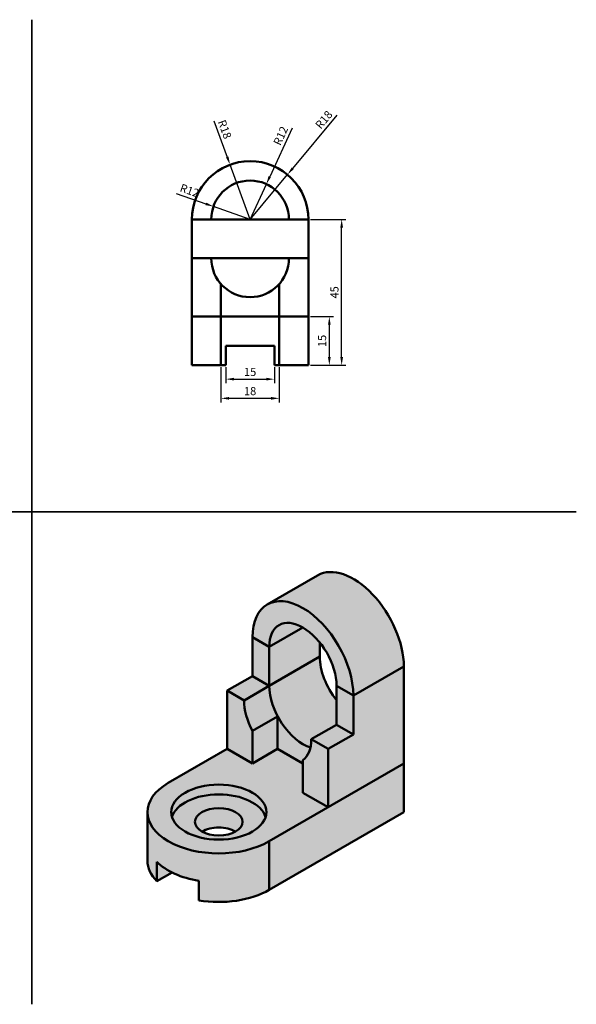
# Model space of a CAD drawing. Units: millimetres. Extents: x 2643 to 3341, y 1496 to 1804.
# Tile 1 of 2: x 2815 to 2987, y 1500 to 1804. Entities that reach past the tile are written whole.
import ezdxf

# ---------------------------------------------------------------- set-up
doc = ezdxf.new("R2010")
doc.units = ezdxf.units.MM
for name, color, linetype, lineweight in [('M-DIMS', 2, 'Continuous', 25), ('M-HATC', 252, 'Continuous', 18), ('M-OUTL', 7, 'Continuous', 50), ('M-TTLB', 8, 'Continuous', 35)]:
    doc.layers.add(name, color=color, linetype=linetype, lineweight=lineweight)
doc.styles.get("Standard").update_dxf_attribs({"font": 'arial.ttf'})
doc.dimstyles.new('ISO-25', dxfattribs={"dimtxt": 2.5, "dimasz": 2.5, "dimexe": 1.25, "dimexo": 0.625, "dimtad": 1, "dimtxsty": 'Standard', "dimcen": 2.5, "dimadec": 0, "dimazin": 0, "dimtfac": 1, "dimtmove": 0, "dimatfit": 3, "dimfxl": 1, "dimarcsym": 0})

# ---------------------------------------------------------------- blocks, each defined once
blk = doc.blocks.new('*D8')
at = {"layer": 'Defpoints', "color": 0, "transparency": 16777216}
for p in [(2878.539861946249, 1697.12622113536), (2893.539861946249, 1697.12622113536), (2893.539861946249, 1692.828022005697)]:
    blk.add_point(p, dxfattribs=at)
at = {"layer": 'M-DIMS', "color": 0, "lineweight": -2, "transparency": 16777216}
for p, q in [((2878.539861946249, 1696.50122113536), (2878.539861946249, 1691.578022005697)), ((2893.539861946249, 1696.50122113536), (2893.539861946249, 1691.578022005697)), ((2881.039861946249, 1692.828022005697), (2891.039861946249, 1692.828022005697))]:
    blk.add_line(p, q, dxfattribs=at)
at = {"layer": 'M-DIMS', "color": 0, "transparency": 16777216}
for points in [[(2881.039861946249, 1693.244688672364), (2881.039861946249, 1692.41135533903), (2878.539861946249, 1692.828022005697)], [(2891.039861946249, 1693.244688672364), (2891.039861946249, 1692.41135533903), (2893.539861946249, 1692.828022005697)]]:
    blk.add_solid(points, dxfattribs=at)
at = {"layer": 'M-DIMS', "color": 0, "transparency": 16777216, "insert": (2886.039861946249, 1694.729454475001), "char_height": 2.5, "attachment_point": 5}
blk.add_mtext('15', dxfattribs=at)
blk = doc.blocks.new('*D9')
at = {"layer": 'Defpoints', "color": 0, "transparency": 16777216}
for p in [(2877.039861946249, 1697.12622113536), (2895.039861946249, 1697.12622113536), (2895.039861946249, 1686.907164766469)]:
    blk.add_point(p, dxfattribs=at)
at = {"layer": 'M-DIMS', "color": 0, "lineweight": -2, "transparency": 16777216}
for p, q in [((2877.039861946249, 1696.50122113536), (2877.039861946249, 1685.657164766469)), ((2895.039861946249, 1696.50122113536), (2895.039861946249, 1685.657164766469)), ((2879.539861946249, 1686.907164766469), (2892.539861946249, 1686.907164766469))]:
    blk.add_line(p, q, dxfattribs=at)
at = {"layer": 'M-DIMS', "color": 0, "transparency": 16777216}
for points in [[(2879.539861946249, 1687.323831433136), (2879.539861946249, 1686.490498099803), (2877.039861946249, 1686.907164766469)], [(2892.539861946249, 1687.323831433136), (2892.539861946249, 1686.490498099803), (2895.039861946249, 1686.907164766469)]]:
    blk.add_solid(points, dxfattribs=at)
at = {"layer": 'M-DIMS', "color": 0, "transparency": 16777216, "insert": (2886.039861946249, 1688.808597235774), "char_height": 2.5, "attachment_point": 5}
blk.add_mtext('18', dxfattribs=at)
blk = doc.blocks.new('*D10')
at = {"layer": 'Defpoints', "color": 0, "transparency": 16777216}
for p in [(2904.03986194625, 1712.126221135361), (2910.511864211038, 1712.126221135361), (2904.03986194625, 1697.126221135361)]:
    blk.add_point(p, dxfattribs=at)
at = {"layer": 'M-DIMS', "color": 0, "lineweight": -2, "transparency": 16777216}
for p, q in [((2904.66486194625, 1712.126221135361), (2911.761864211038, 1712.126221135361)), ((2910.511864211038, 1699.626221135361), (2910.511864211038, 1709.626221135361)), ((2904.66486194625, 1697.126221135361), (2911.761864211038, 1697.126221135361))]:
    blk.add_line(p, q, dxfattribs=at)
at = {"layer": 'M-DIMS', "color": 0, "transparency": 16777216}
for points in [[(2910.095197544371, 1709.626221135361), (2910.928530877704, 1709.626221135361), (2910.511864211038, 1712.126221135361)], [(2910.095197544371, 1699.626221135361), (2910.928530877704, 1699.626221135361), (2910.511864211038, 1697.126221135361)]]:
    blk.add_solid(points, dxfattribs=at)
at = {"layer": 'M-DIMS', "color": 0, "transparency": 16777216, "insert": (2908.610431741733, 1704.626221135359), "char_height": 2.5, "attachment_point": 5, "rotation": 90}
blk.add_mtext('15', dxfattribs=at)
blk = doc.blocks.new('*D11')
at = {"layer": 'Defpoints', "color": 0, "transparency": 16777216}
for p in [(2904.03986194625, 1742.126221135361), (2914.32004968833, 1742.126221135361), (2904.03986194625, 1697.126221135361)]:
    blk.add_point(p, dxfattribs=at)
at = {"layer": 'M-DIMS', "color": 0, "lineweight": -2, "transparency": 16777216}
for p, q in [((2904.66486194625, 1742.126221135361), (2915.57004968833, 1742.126221135361)), ((2914.32004968833, 1699.626221135361), (2914.32004968833, 1739.626221135361)), ((2904.66486194625, 1697.126221135361), (2915.57004968833, 1697.126221135361))]:
    blk.add_line(p, q, dxfattribs=at)
at = {"layer": 'M-DIMS', "color": 0, "transparency": 16777216}
for points in [[(2913.903383021663, 1739.626221135361), (2914.736716354996, 1739.626221135361), (2914.32004968833, 1742.126221135361)], [(2913.903383021663, 1699.626221135361), (2914.736716354996, 1699.626221135361), (2914.32004968833, 1697.126221135361)]]:
    blk.add_solid(points, dxfattribs=at)
at = {"layer": 'M-DIMS', "color": 0, "transparency": 16777216, "insert": (2912.423733180827, 1719.626221135359), "char_height": 2.5, "attachment_point": 5, "rotation": 90}
blk.add_mtext('45', dxfattribs=at)
blk = doc.blocks.new('*D12')
at = {"layer": 'Defpoints', "color": 0, "transparency": 16777216}
for p in [(2897.568460366327, 1755.9498031049), (2886.039861946246, 1742.126221135359)]:
    blk.add_point(p, dxfattribs=at)
at = {"layer": 'M-DIMS', "color": 0, "lineweight": -2, "transparency": 16777216}
for p, q in [((2912.838621649522, 1774.259776138453), (2899.169654591339, 1757.869745045113)), ((2886.039861946246, 1742.126221135359), (2897.568460366327, 1755.9498031049))]:
    blk.add_line(p, q, dxfattribs=at)
at = {"layer": 'M-DIMS', "color": 0, "transparency": 16777216}
blk.add_solid([(2898.849664267969, 1758.136610749282), (2899.489644914707, 1757.602879340945), (2897.568460366327, 1755.9498031049)], dxfattribs=at)
at = {"layer": 'M-DIMS', "color": 0, "transparency": 16777216, "insert": (2909.063405808288, 1772.701805209806), "char_height": 2.5, "attachment_point": 5, "rotation": 50.172551131776245}
blk.add_mtext('R18', dxfattribs=at)
blk = doc.blocks.new('*D13')
at = {"layer": 'Defpoints', "color": 0, "transparency": 16777216}
for p in [(2891.051977523317, 1753.029371938779), (2886.039861946248, 1742.126221135359)]:
    blk.add_point(p, dxfattribs=at)
at = {"layer": 'M-DIMS', "color": 0, "lineweight": -2, "transparency": 16777216}
for p, q in [((2898.991408479002, 1770.300484640011), (2892.09616826854, 1755.300861689492)), ((2886.039861946248, 1742.126221135359), (2891.051977523317, 1753.029371938779))]:
    blk.add_line(p, q, dxfattribs=at)
at = {"layer": 'M-DIMS', "color": 0, "transparency": 16777216}
blk.add_solid([(2891.717586643421, 1755.474893480363), (2892.474749893659, 1755.126829898622), (2891.051977523317, 1753.029371938779)], dxfattribs=at)
at = {"layer": 'M-DIMS', "color": 0, "transparency": 16777216, "insert": (2895.779892777806, 1767.815655975434), "char_height": 2.5, "attachment_point": 5, "rotation": 65.31203083876427}
blk.add_mtext('R12', dxfattribs=at)
blk = doc.blocks.new('*D35')
at = {"layer": 'Defpoints', "color": 0, "transparency": 16777216}
for p in [(2879.838123, 1759.024104), (2886.039862, 1742.126221)]:
    blk.add_point(p, dxfattribs=at)
at = {"layer": 'M-DIMS', "color": 0, "lineweight": -2, "transparency": 16777216}
for p, q in [((2874.871761228464, 1772.555953720068), (2878.976770383051, 1761.371032134664)), ((2886.039862, 1742.126221), (2879.838123, 1759.024104))]:
    blk.add_line(p, q, dxfattribs=at)
at = {"layer": 'M-DIMS', "color": 0, "transparency": 16777216}
blk.add_solid([(2879.367925072162, 1761.514590904155), (2878.585615693941, 1761.227473365172), (2879.838123, 1759.024104)], dxfattribs=at)
at = {"layer": 'M-DIMS', "color": 0, "transparency": 16777216, "insert": (2877.902089838132, 1769.817955075101), "char_height": 2.5, "attachment_point": 5, "rotation": 290.1537820808809}
blk.add_mtext('R18', dxfattribs=at)
blk = doc.blocks.new('*D36')
at = {"layer": 'Defpoints', "color": 0, "transparency": 16777216}
for p in [(2874.721666, 1746.113505), (2886.039862000001, 1742.126221)]:
    blk.add_point(p, dxfattribs=at)
at = {"layer": 'M-DIMS', "color": 0, "lineweight": -2, "transparency": 16777216}
for p, q in [((2863.216570279684, 1750.16663184849), (2872.363708454077, 1746.944189182844)), ((2886.039862000001, 1742.126221), (2874.721666, 1746.113505))]:
    blk.add_line(p, q, dxfattribs=at)
at = {"layer": 'M-DIMS', "color": 0, "transparency": 16777216}
blk.add_solid([(2872.502155817885, 1747.337182107165), (2872.22526109027, 1746.551196258524), (2874.721666, 1746.113505)], dxfattribs=at)
at = {"layer": 'M-DIMS', "color": 0, "transparency": 16777216, "insert": (2867.235873630472, 1750.744046054824), "char_height": 2.5, "attachment_point": 5, "rotation": 340.59316357138516}
blk.add_mtext('R12', dxfattribs=at)

msp = doc.modelspace()

# ---------------------------------------------------------------- hatches: boundary and pattern name
at = {"layer": 'M-HATC'}
h = msp.add_hatch(color=256, dxfattribs=at)
h.dxf.hatch_style = 1
h.paths.add_polyline_path([(2933.516942481301, 1604.176370603883), (2917.92848521322, 1595.176370603883), (2917.92848521322, 1583.176370603883), (2910.134256579122, 1578.676370603883), (2910.134256579238, 1560.676370603955), (2933.516942481301, 1574.176370603883)])
h.paths.add_polyline_path([(2933.516942481301, 1574.176370603883), (2910.134256579238, 1560.676370603955), (2891.947723099637, 1550.176370603883), (2891.947723099637, 1535.176370603883), (2933.516942481301, 1559.176370603883)])
edge = h.paths.add_edge_path()
edge.add_line((2910.134256579169, 1560.676370603914), (2902.340027945024, 1565.176370603942))
edge.add_line((2902.340027945024, 1565.176370603942), (2902.340027945024, 1574.176370604203))
edge.add_line((2902.340027945024, 1574.176370604203), (2894.545799311216, 1578.676370604033))
edge.add_line((2894.545799311216, 1578.676370604033), (2886.75157067706, 1574.176370603912))
edge.add_line((2886.75157067706, 1574.176370603912), (2878.957342042936, 1578.676370603927))
edge.add_line((2878.957342042936, 1578.676370603927), (2860.770808564148, 1568.176370604339))
edge.add_ellipse((2876.359265831439, 1559.176370603883), major_axis=(-22.04540768513047, 0), ratio=0.5773502691893942, start_angle=150.0000000000131, end_angle=329.99999999998147, ccw=False)
edge.add_line((2891.947723099778, 1550.176370603965), (2910.134256579169, 1560.676370603914))
edge = h.paths.add_edge_path()
edge.add_ellipse((2876.359265831439, 1559.176370603883), major_axis=(-22.04540768513047, 0), ratio=0.5773502691893942, start_angle=0, end_angle=150.0000000000124, ccw=False)
edge.add_line((2854.313858146337, 1559.176370603687), (2854.313858146337, 1544.176370603629))
edge.add_ellipse((2876.359265831439, 1544.176370603883), major_axis=(-22.04540768513047, 0), ratio=0.5773502691893942, start_angle=360, end_angle=378.3086229740257)
edge.add_line((2857.232362851408, 1537.847558645967), (2857.232362851408, 1543.847558645968))
edge.add_ellipse((2876.359265831439, 1550.176370603883), major_axis=(-22.04540768513047, 0), ratio=0.5773502691893942, start_angle=378.3086229740257, end_angle=393.6807393147395)
edge.add_ellipse((2876.359265831439, 1550.176370603883), major_axis=(-22.04540768513047, 0), ratio=0.5773502691893942, start_angle=393.6807393147395, end_angle=423.3447265862672)
edge.add_line((2870.222743908083, 1537.951490254265), (2870.222743908083, 1531.951490254265))
edge.add_ellipse((2876.359265831439, 1544.176370603883), major_axis=(-22.04540768513047, 0), ratio=0.5773502691893942, start_angle=423.3447265862672, end_angle=510.0000000000425)
edge.add_line((2891.947723099637, 1535.176370603864), (2891.947723099637, 1550.176370603863))
edge = h.paths.add_edge_path()
edge.add_ellipse((2876.359265831439, 1559.176370603883), major_axis=(-22.04540768513047, 0), ratio=0.5773502691893942, start_angle=0, end_angle=150.0000000000123)
edge.add_ellipse((2876.359265831439, 1559.176370603883), major_axis=(-22.04540768513047, 0), ratio=0.5773502691893942, start_angle=150.0000000000123, end_angle=329.9999999999814)
edge.add_ellipse((2876.359265831439, 1559.176370603883), major_axis=(-22.04540768513047, 0), ratio=0.5773502691893942, start_angle=329.9999999999814, end_angle=360)
edge = h.paths.add_edge_path(flags=16)
edge.add_ellipse((2876.359265831439, 1559.176370603883), major_axis=(-14.69693845669906, 0), ratio=0.5773502691902185, start_angle=5.920136941275302, end_angle=174.0798630587249, ccw=False)
edge.add_ellipse((2876.359265831439, 1559.176370603883), major_axis=(-14.69693845669906, 0), ratio=0.5773502691902185, start_angle=174.0798630587249, end_angle=365.92013694127525, ccw=False)
edge = h.paths.add_edge_path(flags=0)
edge.add_ellipse((2876.359265831439, 1556.176370603883), major_axis=(-7.348469228349532, 0), ratio=0.5773502691902185, start_angle=0, end_angle=360)
h.paths.add_polyline_path([(2894.545799311274, 1588.73911667028), (2886.75157067706, 1584.239116670192), (2886.75157067706, 1574.176370603912), (2894.545799311274, 1578.676370604067)])
edge = h.paths.add_edge_path()
edge.add_ellipse((2894.545799310925, 1587.676370603796), major_axis=(7.348469228327981, -12.72792206133827), ratio=0.5773502691919116, start_angle=210.0000000002129, end_angle=263.79747378773834, ccw=False)
edge.add_line((2884.153494465513, 1593.676370603782), (2878.957342042961, 1596.676370603883))
edge.add_line((2878.957342042961, 1596.676370603883), (2878.957342042961, 1578.676370603913))
edge.add_line((2878.957342042961, 1578.676370603913), (2886.75157067706, 1574.176370603912))
edge.add_line((2886.75157067706, 1574.176370603912), (2886.75157067706, 1584.2391166702))
edge = h.paths.add_edge_path()
edge.add_line((2910.134256579122, 1578.676370603883), (2904.938104156335, 1581.676370603783))
edge.add_ellipse((2894.545799310925, 1587.676370603796), major_axis=(7.348469228327981, -12.72792206133827), ratio=0.5773502691919116, start_angle=379.85756861646945, end_angle=389.9999999999722, ccw=False)
edge.add_ellipse((2894.545799310925, 1587.676370603796), major_axis=(7.348469228327981, -12.72792206133827), ratio=0.5773502691919116, start_angle=362.0747159111078, end_angle=379.85756861646945, ccw=False)
edge.add_line((2902.340027945024, 1575.239116670666), (2902.340027945024, 1565.176370603942))
edge.add_line((2902.340027945024, 1565.176370603942), (2910.134256579238, 1560.676370603874))
edge.add_line((2910.134256579238, 1560.676370603874), (2910.134256579122, 1578.676370603883))
h.paths.add_polyline_path([(2917.92848521322, 1583.176370603883), (2912.732332790527, 1586.176370603883), (2904.938104156304, 1581.676370603801), (2910.134256579122, 1578.676370603883)])
h.paths.add_polyline_path([(2891.947723099804, 1598.176370603854), (2886.75157067706, 1601.176370603883), (2878.957342042961, 1596.676370603883), (2884.153494465538, 1593.676370603767)])
h.paths.add_polyline_path([(2891.947723099753, 1610.176370603883), (2886.75157067706, 1613.176370603883), (2886.75157067706, 1601.176370603883), (2891.947723099753, 1598.176370603883)], flags=17)
edge = h.paths.add_edge_path()
edge.add_ellipse((2902.34002794514, 1604.176370603883), major_axis=(7.348469228327981, -12.72792206133827), ratio=0.5773502691919116, start_angle=510.0000000000128, end_angle=569.999999999972, ccw=False)
edge.add_ellipse((2902.34002794514, 1604.176370603883), major_axis=(7.348469228327981, -12.72792206133827), ratio=0.5773502691919116, start_angle=474.8960906392445, end_angle=510.0000000000128, ccw=False)
edge.add_ellipse((2902.34002794514, 1604.176370603883), major_axis=(7.348469228327981, -12.72792206133827), ratio=0.5773502691919116, start_angle=389.9999999999722, end_angle=474.8960906392445, ccw=False)
edge.add_line((2912.73233279055, 1598.17637060387), (2917.928485213233, 1595.176370603877))
edge.add_ellipse((2902.34002794514, 1604.176370603883), major_axis=(11.02270384251673, -19.09188309199311), ratio=0.5773502691892949, start_angle=29.99999999989788, end_angle=180.0000000000081)
edge.add_ellipse((2902.34002794514, 1604.176370603883), major_axis=(11.02270384251673, -19.09188309199311), ratio=0.5773502691892949, start_angle=180.0000000000081, end_angle=209.9999999998979)
edge.add_line((2886.751570677047, 1613.17637060389), (2891.947723099729, 1610.176370603897))
h.paths.add_polyline_path([(2917.92848521322, 1595.176370603883), (2912.732332790527, 1598.176370603883), (2912.732332790527, 1586.176370603883), (2917.92848521322, 1583.176370603883)], flags=17)
edge = h.paths.add_edge_path()
edge.add_ellipse((2917.92848521322, 1613.176370603883), major_axis=(11.02270384251673, -19.09188309199311), ratio=0.5773502691892949, start_angle=29.99999999989788, end_angle=180)
edge.add_line((2906.905781370834, 1632.268253695929), (2891.317324102751, 1623.268253695927))
edge.add_ellipse((2902.34002794514, 1604.176370603883), major_axis=(11.02270384251673, -19.09188309199311), ratio=0.5773502691892949, start_angle=29.99999999989791, end_angle=180.0000000000082, ccw=False)
edge.add_line((2917.928485213232, 1595.17637060389), (2933.516942481312, 1604.17637060389))
edge = h.paths.add_edge_path(flags=17)
edge.add_ellipse((2876.359265831439, 1550.176370603883), major_axis=(-22.04540768513047, 0), ratio=0.5773502691893942, start_angle=378.3086229740258, end_angle=393.6807393147396, ccw=False)
edge.add_line((2857.232362851408, 1543.847558645968), (2857.232362851408, 1537.847558645975))
edge.add_line((2857.232362851408, 1537.847558645975), (2861.92424961148, 1540.556420729916))
edge = h.paths.add_edge_path()
edge.add_ellipse((2894.545799310925, 1587.676370603796), major_axis=(7.348469228327981, -12.72792206133827), ratio=0.5773502691919116, start_angle=362.0747159111078, end_angle=379.8575686164694)
edge.add_ellipse((2902.34002794514, 1592.176370603883), major_axis=(7.348469228327981, -12.72792206133827), ratio=0.5773502691919116, start_angle=263.79747378769656, end_angle=340.14243138353595, ccw=False)
edge.add_line((2894.545799311274, 1588.739116670287), (2894.545799311274, 1578.676370604))
edge.add_line((2894.545799311274, 1578.676370604), (2902.340027945024, 1574.176370604203))
edge.add_line((2902.340027945024, 1574.176370604203), (2902.340027945024, 1575.239116670666))
h = msp.add_hatch(color=256, dxfattribs=at)
h.dxf.hatch_style = 1
edge = h.paths.add_edge_path()
edge.add_ellipse((2902.34002794514, 1592.176370603883), major_axis=(7.348469228327981, -12.72792206133827), ratio=0.5773502691919116, start_angle=210.0000000002129, end_angle=263.79747378769656, ccw=False)
edge.add_line((2891.947723099731, 1598.176370603812), (2884.153494465514, 1593.676370603753))
edge.add_ellipse((2894.545799310925, 1587.676370603796), major_axis=(7.348469228327981, -12.72792206133827), ratio=0.5773502691919116, start_angle=210.0000000002128, end_angle=263.7974737877383)
edge.add_line((2886.751570677063, 1584.239116670194), (2894.545799311277, 1588.739116670281))
edge = h.paths.add_edge_path()
edge.add_ellipse((2917.92848521322, 1601.176370603883), major_axis=(7.348469228327981, -12.72792206133827), ratio=0.5773502691919116, start_angle=210.0000000002129, end_angle=294.89609063918937, ccw=False)
edge.add_line((2907.53618036781, 1607.176370603841), (2891.947723099728, 1598.176370603869))
edge.add_ellipse((2902.34002794514, 1592.176370603883), major_axis=(7.348469228327981, -12.72792206133827), ratio=0.5773502691919116, start_angle=210.0000000002128, end_angle=263.7974737876965)
edge.add_ellipse((2902.34002794514, 1592.176370603883), major_axis=(7.348469228327981, -12.72792206133827), ratio=0.5773502691919116, start_angle=263.7974737876965, end_angle=340.142431383536)
edge.add_ellipse((2894.545799310925, 1587.676370603796), major_axis=(7.348469228327981, -12.72792206133827), ratio=0.5773502691919116, start_angle=379.8575686164694, end_angle=389.9999999999722)
edge.add_line((2904.938104156336, 1581.676370603819), (2912.732332790527, 1586.176370603883))
edge.add_line((2912.732332790527, 1586.176370603883), (2912.732332790527, 1593.784065758426))
edge = h.paths.add_edge_path()
edge.add_line((2907.536180367833, 1607.176370603854), (2907.536180367833, 1611.568675449341))
edge.add_ellipse((2902.34002794514, 1604.176370603883), major_axis=(7.348469228327981, -12.72792206133827), ratio=0.5773502691919116, start_angle=474.8960906392444, end_angle=510.0000000000128)
edge.add_line((2902.340027945145, 1616.176370603886), (2891.947723099753, 1610.176370603883))
edge.add_line((2891.947723099753, 1610.176370603883), (2891.947723099753, 1598.176370603883))
edge.add_line((2891.947723099753, 1598.176370603883), (2907.536180367833, 1607.176370603854))
edge = h.paths.add_edge_path()
edge.add_ellipse((2902.34002794514, 1604.176370603883), major_axis=(7.348469228327981, -12.72792206133827), ratio=0.5773502691919116, start_angle=510.0000000000128, end_angle=209.9999999999721)
edge.add_line((2891.947723099728, 1610.176370603869), (2902.340027945145, 1616.176370603886))
edge = h.paths.add_edge_path()
edge.add_ellipse((2876.359265831439, 1559.176370603883), major_axis=(-14.69693845669906, 0), ratio=0.5773502691902185, start_angle=174.0798630587248, end_angle=365.9201369412752)
edge.add_ellipse((2876.359265831439, 1556.176370603883), major_axis=(-14.69693845669906, 0), ratio=0.5773502691902185, start_angle=185.9201369408757, end_angle=354.0798630591243, ccw=False)
edge = h.paths.add_edge_path()
edge.add_ellipse((2876.359265831439, 1556.176370603883), major_axis=(-14.69693845669906, 0), ratio=0.5773502691902185, start_angle=185.9201369408757, end_angle=354.0798630591242)
edge.add_ellipse((2876.359265831439, 1559.176370603883), major_axis=(-14.69693845669906, 0), ratio=0.5773502691902185, start_angle=5.920136941275217, end_angle=174.0798630587248)
edge = h.paths.add_edge_path(flags=16)
edge.add_ellipse((2876.359265831439, 1556.176370603883), major_axis=(-7.348469228349532, 0), ratio=0.5773502691902185, start_angle=0, end_angle=360)
h = msp.add_hatch(color=256, dxfattribs=at)
h.dxf.hatch_style = 1
edge = h.paths.add_edge_path()
edge.add_ellipse((2876.359265831439, 1550.176370603883), major_axis=(-7.348469228349532, 0), ratio=0.5773502691902185, start_angle=569.9999999999732, end_angle=690.0000000000268, ccw=False)
edge.add_ellipse((2876.359265831439, 1556.176370603883), major_axis=(-7.348469228349532, 0), ratio=0.5773502691902185, start_angle=149.9999999999745, end_angle=390.0000000000255)

# ---------------------------------------------------------------- linework, layer by layer
at = {"layer": 'M-OUTL'}
for p, q in [((2868.039861946249, 1712.12622113536), (2868.039861946249, 1742.12622113536)), ((2868.039861946249, 1742.12622113536), (2904.039861946248, 1742.12622113536)), ((2904.039861946248, 1742.12622113536), (2904.039861946248, 1712.12622113536)), ((2868.039861946249, 1730.12622113536), (2904.039861946248, 1730.12622113536)), ((2877.039861946249, 1722.188967202166), (2877.039861946249, 1697.12622113536)), ((2895.039861946249, 1722.188967202166), (2895.039861946249, 1697.12622113536)), ((2868.039861946249, 1697.12622113536), (2868.039861946249, 1712.12622113536)), ((2868.039861946249, 1712.12622113536), (2904.039861946248, 1712.12622113536)), ((2904.039861946248, 1712.12622113536), (2904.039861946248, 1697.12622113536)), ((2886.039861946249, 1703.12622113536), (2878.539861946249, 1703.12622113536)), ((2878.539861946249, 1703.126221135359), (2878.539861946249, 1697.12622113536)), ((2886.039861946249, 1703.12622113536), (2893.539861946249, 1703.12622113536)), ((2893.539861946249, 1703.126221135359), (2893.539861946249, 1697.12622113536)), ((2868.039861946249, 1697.12622113536), (2878.539861946248, 1697.12622113536)), ((2893.539861946249, 1697.12622113536), (2904.039861946248, 1697.12622113536)), ((2906.905781370728, 1632.268253695867), (2891.317324102647, 1623.268253695867)), ((2891.947723099753, 1610.176370603883), (2902.34002794514, 1616.176370603883)), ((2886.75157067706, 1613.176370603883), (2891.947723099753, 1610.176370603883)), ((2886.75157067706, 1601.176370603883), (2886.75157067706, 1613.176370603883)), ((2907.536180367833, 1611.568675449329), (2907.536180367833, 1607.176370603854)), ((2891.947723099753, 1610.176370603883), (2891.947723099753, 1598.176370603883)), ((2891.947723099753, 1598.176370603883), (2907.536180367833, 1607.176370603854)), ((2933.516942481301, 1604.176370603883), (2917.92848521322, 1595.176370603883)), ((2933.516942481301, 1559.176370603883), (2933.516942481301, 1604.176370603883)), ((2886.75157067706, 1601.176370603883), (2878.957342042961, 1596.676370603883)), ((2891.947723099753, 1598.176370603883), (2886.75157067706, 1601.176370603883)), ((2878.957342042961, 1596.676370603883), (2878.957342042961, 1578.676370603912)), ((2884.153494465538, 1593.676370603767), (2878.957342042961, 1596.676370603883)), ((2884.153494465538, 1593.676370603767), (2891.947723099753, 1598.176370603825)), ((2917.92848521322, 1595.176370603883), (2912.732332790527, 1598.176370603883)), ((2912.732332790527, 1586.176370603883), (2912.732332790527, 1598.176370603883)), ((2917.92848521322, 1595.176370603883), (2917.92848521322, 1583.176370603883)), ((2886.75157067706, 1584.239116670192), (2894.545799311274, 1588.73911667028)), ((2894.545799311274, 1588.73911667028), (2894.545799311274, 1578.676370604)), ((2886.75157067706, 1574.176370603912), (2886.75157067706, 1584.239116670192)), ((2912.732332790527, 1586.176370603883), (2904.938104156196, 1581.676370603738)), ((2917.92848521322, 1583.176370603883), (2912.732332790527, 1586.176370603883)), ((2910.134256579122, 1578.676370603883), (2904.938104156312, 1581.676370603796)), ((2917.92848521322, 1583.176370603883), (2910.134256579122, 1578.676370603883)), ((2878.957342042961, 1578.676370603942), (2860.770808563359, 1568.176370603883)), ((2878.957342042961, 1578.676370603912), (2886.75157067706, 1574.176370603912)), ((2886.75157067706, 1574.176370603912), (2894.545799311158, 1578.676370604)), ((2894.545799311274, 1578.676370604), (2902.340027945024, 1574.176370604203)), ((2910.134256579122, 1578.676370603883), (2910.134256579238, 1560.676370603913)), ((2902.340027945024, 1565.176370603942), (2902.340027945024, 1575.239116670658)), ((2933.516942481301, 1574.176370603883), (2891.947723099637, 1550.176370603883)), ((2933.516942481301, 1559.176370603883), (2933.516942481301, 1574.176370603883)), ((2910.134256579122, 1560.676370603942), (2902.340027945024, 1565.176370603942)), ((2854.313858146337, 1559.176370603883), (2854.313858146337, 1544.176370603883)), ((2891.947723099637, 1535.176370603883), (2933.516942481301, 1559.176370603883)), ((2910.134256579238, 1560.676370603942), (2910.134256579122, 1560.676370603942)), ((2891.947723099637, 1550.176370603883), (2891.947723099637, 1535.176370603883)), ((2857.232362851408, 1537.847558645975), (2857.232362851408, 1543.847558645975)), ((2857.232362851408, 1537.847558645975), (2861.924249611469, 1540.55642072991)), ((2857.232362851403, 1537.847558645972), (2857.232362851403, 1537.847558645972)), ((2870.222743908083, 1531.951490254265), (2870.222743908083, 1537.951490254265))]:
    msp.add_line(p, q, dxfattribs=at)
for centre, radius, start, end in [((2886.039861946249, 1742.12622113536), 18, 0, 180), ((2886.039861946249, 1742.12622113536), 12, 0, 180), ((2886.039861946249, 1730.12622113536), 12, 180, 0)]:
    msp.add_arc(centre, radius, start, end, dxfattribs=at)
for centre, major_axis, ratio, start_param, end_param in [((2917.92848521322, 1613.176370603883), (11.02270384251673, -19.09188309199311), 0.5773502691892949, 0.7853981633956768, 3.141592653589793), ((2902.34002794514, 1604.176370603883), (11.02270384251673, -19.09188309199311), 0.5773502691892949, 0.7853981633956768, 3.926990816985469), ((2902.34002794514, 1604.176370603883), (7.348469228327981, -12.72792206133827), 0.5773502691919116, 7.068583470574494, 10.21017612416428), ((2917.92848521322, 1601.176370603883), (7.348469228327981, -12.72792206133827), 0.5773502691919116, 3.926990816989551, 4.974188368187188), ((2902.34002794514, 1592.176370603883), (7.348469228327981, -12.72792206133827), 0.5773502691919116, 3.926990816989551, 5.724195441142849), ((2894.545799310925, 1587.676370603796), (7.348469228327981, -12.72792206133827), 0.5773502691919116, 3.926990816989551, 4.649725064831715), ((2894.545799310925, 1587.676370603796), (7.348469228327981, -12.72792206133827), 0.5773502691919116, 6.3458492227717, 7.068583470574494), ((2876.359265831439, 1559.176370603883), (-22.04540768513047, 0), 0.5773502691893942, 5.497787143783955, 8.63937979737317), ((2876.359265831439, 1556.176370603883), (-14.69693845669906, 0), 0.5773502691902185, 3.319303254432881, 6.105474706336497), ((2876.359265831439, 1550.176370603883), (-7.348469228349532, 0), 0.5773502691902185, 10.21017612416577, 11.78097245096278), ((2876.359265831439, 1544.176370603883), (-22.04540768513047, 0), 0.5773502691893942, 6.283185307179586, 6.803598218721409), ((2876.359265831439, 1550.176370603883), (-22.04540768513047, 0), 0.5773502691893942, 6.803598218721409, 7.571897216845255), ((2876.359265831439, 1544.176370603883), (-22.04540768513047, 0), 0.5773502691893942, 7.571897216845255, 8.63937979737259)]:
    msp.add_ellipse(centre, major_axis=major_axis, ratio=ratio, start_param=start_param, end_param=end_param, dxfattribs=at)
for centre, major_axis in [((2876.359265831439, 1559.176370603883), (-14.69693845669906, 0)), ((2876.359265831439, 1556.176370603883), (-7.348469228349532, 0))]:
    msp.add_ellipse(centre, major_axis=major_axis, ratio=0.5773502691902185, dxfattribs=at)
at = {"layer": 'M-TTLB'}
for p, q in [((2818.579943598263, 1803.781093318395), (2818.579943598263, 1499.861899971862)), ((2818.579943598263, 1651.821496645129), (2651.296863881127, 1651.821496645129)), ((2818.579943598263, 1651.821496645129), (2986.808116079883, 1651.821496645129))]:
    msp.add_line(p, q, dxfattribs=at)

# ---------------------------------------------------------------- dimensions: what is measured, and where the dimension line sits
at = {"layer": 'M-DIMS'}
for center, mpoint, override, picture, middle in [((2886.039861946246, 1742.126221135359), (2897.568460366327, 1755.9498031049), {"dimclrd": 0, "dimclre": 0, "dimclrt": 0}, '*D12', (2910.523661786008, 1771.483980134167)), ((2886.039862, 1742.126221), (2879.838123, 1759.024104), {"dimdec": 0, "dimlfac": 1, "dimrnd": 0, "dimzin": 0, "dimdsep": 46, "dimlunit": 2}, '*D35', (2876.117079694783, 1769.162833541747)), ((2886.039861946248, 1742.126221135359), (2891.051977523317, 1753.029371938779), {"dimclrd": 0, "dimclre": 0, "dimclrt": 0}, '*D13', (2897.488158432759, 1767.030376100531))]:
    dim = msp.add_radius_dim(center=center, mpoint=mpoint, dimstyle='ISO-25', override=override, dxfattribs=at)
    dim.commit()
    dim.dimension.update_dxf_attribs({"geometry": picture, "text_midpoint": middle, "dimtype": 164})
dim = msp.add_radius_dim(center=(2886.039862000001, 1742.126221), mpoint=(2874.721666, 1746.113505), dimstyle='ISO-25', override={"dimdec": 0, "dimlfac": 1, "dimrnd": 0, "dimzin": 0, "dimdsep": 46, "dimlunit": 2}, dxfattribs=at)
dim.commit()
dim.dimension.update_dxf_attribs({"geometry": '*D36', "text_midpoint": (2867.235873630472, 1750.744046054824)})
for base, p2, picture, middle in [((2914.32004968833, 1742.126221135361), (2904.039861946248, 1742.12622113536), '*D11', (2912.423733180827, 1719.626221135359)), ((2910.511864211038, 1712.126221135361), (2904.039861946248, 1712.12622113536), '*D10', (2908.610431741733, 1704.626221135359))]:
    dim = msp.add_linear_dim(base=base, p1=(2904.039861946248, 1697.12622113536), p2=p2, angle=90, dimstyle='ISO-25', override={"dimclrd": 0, "dimclre": 0, "dimclrt": 0}, dxfattribs=at)
    dim.commit()
    dim.dimension.update_dxf_attribs({"geometry": picture, "text_midpoint": middle})
for base, p1, p2, picture, middle in [((2895.039861946249, 1686.907164766469), (2877.039861946249, 1697.12622113536), (2895.039861946249, 1697.12622113536), '*D9', (2886.039861946249, 1688.808597235774)), ((2893.539861946249, 1692.828022005697), (2878.539861946249, 1697.12622113536), (2893.539861946249, 1697.12622113536), '*D8', (2886.039861946249, 1694.729454475001))]:
    dim = msp.add_linear_dim(base=base, p1=p1, p2=p2, dimstyle='ISO-25', override={"dimclrd": 0, "dimclre": 0, "dimclrt": 0}, dxfattribs=at)
    dim.commit()
    dim.dimension.update_dxf_attribs({"geometry": picture, "text_midpoint": middle})

doc.saveas('drawing.dxf')
